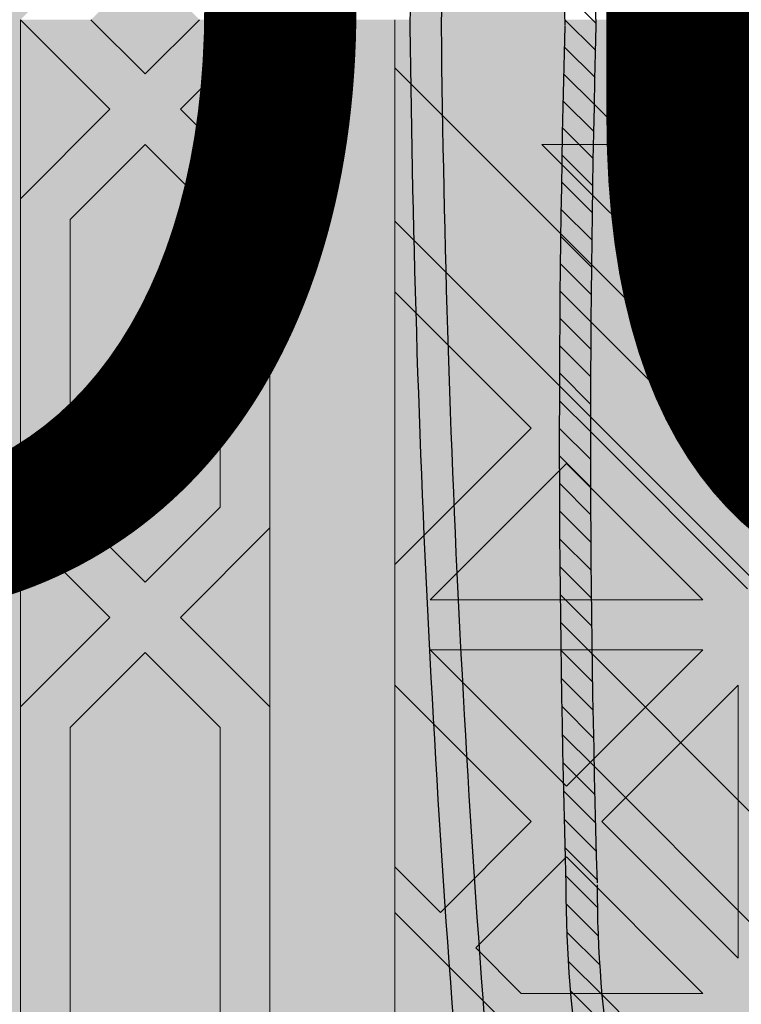
# Model space of a CAD drawing. Units: inches. Extents: x 844 to 2234, y 346 to 1084.
# Tile 71 of 93: x 1997.478 to 2001.166, y 696.335 to 701.365. Entities that reach past the tile are written whole.
import ezdxf

# ---------------------------------------------------------------- set-up
doc = ezdxf.new("R2010")
doc.units = ezdxf.units.IN
doc.header["$MEASUREMENT"] = 0
for name, color, linetype, lineweight in [('A-ANNO-DIMS', 2, 'Continuous', 18), ('furniture', 8, 'Continuous', 18), ('RA-AP-01$0$INT', 35, 'Continuous', 5)]:
    doc.layers.add(name, color=color, linetype=linetype, lineweight=lineweight)
doc.layers.add('RA-AP-01$0$FURN', color=3, linetype='Continuous')
doc.layers.add('RA-AP-01$0$WOOD', color=64, linetype='Continuous')
doc.styles.get("Standard").update_dxf_attribs({"font": 'arial.ttf'})
doc.dimstyles.get("Standard").update_dxf_attribs({"dimtxt": 6, "dimasz": 3, "dimexe": 0.18, "dimexo": 0.0625, "dimgap": 0.09, "dimtad": 0, "dimtih": 1, "dimtoh": 1, "dimdec": 1, "dimzin": 0, "dimdsep": 46, "dimlunit": 3, "dimtxsty": 'Standard', "dimblk": 'ARCHTICK', "dimcen": 0.09, "dimadec": 0, "dimazin": 0, "dimtfac": 1, "dimtdec": 1, "dimtofl": 0, "dimtmove": 0, "dimatfit": 3, "dimfxl": 1, "dimtolj": 1, "dimtzin": 0, "dimarcsym": 0})

# ---------------------------------------------------------------- blocks, each defined once
blk = doc.blocks.new('A$C18D01794')
at = {"layer": 'RA-AP-01$0$INT'}
h = blk.add_hatch(color=256, dxfattribs=at)
h.paths.add_polyline_path([(4.35521, -6.15671), (4.35521, -8.05671), (5.45521, -8.05671), (5.45521, -6.15671)])
h.paths.add_polyline_path([(4.40521, -8.00671), (4.40521, -6.20671), (5.40521, -6.20671), (5.40521, -8.00671)], flags=16)
h = blk.add_hatch(color=256, dxfattribs=at)
h.paths.add_polyline_path([(4.46935, -7.07085), (4.50521, -7.035), (4.50521, -7.10671)])
h.paths.add_polyline_path([(4.45521, -7.085), (4.47692, -7.10671), (4.43349, -7.10671)])
h.paths.add_polyline_path([(4.40521, -7.035), (4.44106, -7.07085), (4.40521, -7.10671)])
h.paths.add_polyline_path([(4.42521, -6.91146), (4.45521, -6.88146), (4.48521, -6.91146), (4.48521, -7.02671), (4.45521, -7.05671), (4.42521, -7.02671)])
h.paths.add_polyline_path([(4.50521, -6.83146), (4.50521, -6.90318), (4.46935, -6.86732)])
h.paths.add_polyline_path([(4.42521, -6.70793), (4.45521, -6.67793), (4.48521, -6.70793), (4.48521, -6.82318), (4.45521, -6.85318), (4.42521, -6.82318)])
h.paths.add_polyline_path([(4.42521, -6.50439), (4.45521, -6.47439), (4.48521, -6.50439), (4.48521, -6.61964), (4.45521, -6.64964), (4.42521, -6.61964)])
h.paths.add_polyline_path([(4.46935, -6.66378), (4.50521, -6.62793), (4.50521, -6.69964)])
h.paths.add_polyline_path([(4.40521, -6.62793), (4.44106, -6.66378), (4.40521, -6.69964)])
h.paths.add_polyline_path([(4.40521, -6.42439), (4.44106, -6.46025), (4.40521, -6.49611)])
h.paths.add_polyline_path([(4.46935, -6.46025), (4.50521, -6.42439), (4.50521, -6.49611)])
h.paths.add_polyline_path([(4.42521, -6.30085), (4.45521, -6.27085), (4.48521, -6.30085), (4.48521, -6.41611), (4.45521, -6.44611), (4.42521, -6.41611)])
h.paths.add_polyline_path([(4.42521, -6.22671), (4.47106, -6.22671), (4.42521, -6.27257)])
h.paths.add_polyline_path([(4.49935, -6.22671), (4.63606, -6.22671), (4.66606, -6.25671), (4.63606, -6.28671), (4.49935, -6.28671), (4.46935, -6.25671)])
h.paths.add_polyline_path([(4.68021, -6.27085), (4.71606, -6.30671), (4.64435, -6.30671)])
h.paths.add_polyline_path([(4.64435, -6.20671), (4.71606, -6.20671), (4.68021, -6.24257)])
h.paths.add_polyline_path([(4.72435, -6.22671), (4.86106, -6.22671), (4.89106, -6.25671), (4.86106, -6.28671), (4.72435, -6.28671), (4.69435, -6.25671)])
h.paths.add_polyline_path([(4.90521, -6.27085), (4.94106, -6.30671), (4.86935, -6.30671)])
h.paths.add_polyline_path([(4.86935, -6.20671), (4.94106, -6.20671), (4.90521, -6.24257)])
h.paths.add_polyline_path([(4.94935, -6.22671), (5.08606, -6.22671), (5.11606, -6.25671), (5.08606, -6.28671), (4.94935, -6.28671), (4.91935, -6.25671)])
h.paths.add_polyline_path([(5.13021, -6.27085), (5.16606, -6.30671), (5.09435, -6.30671)])
h.paths.add_polyline_path([(5.09435, -6.20671), (5.16606, -6.20671), (5.13021, -6.24257)])
h.paths.add_polyline_path([(5.17435, -6.22671), (5.31106, -6.22671), (5.34106, -6.25671), (5.31106, -6.28671), (5.17435, -6.28671), (5.14435, -6.25671)])
h.paths.add_polyline_path([(5.32521, -6.30085), (5.35521, -6.27085), (5.38521, -6.30085), (5.38521, -6.41611), (5.35521, -6.44611), (5.32521, -6.41611)])
h.paths.add_polyline_path([(5.33935, -6.22671), (5.38521, -6.22671), (5.38521, -6.27257)])
h.paths.add_polyline_path([(5.32521, -6.50439), (5.35521, -6.47439), (5.38521, -6.50439), (5.38521, -6.61964), (5.35521, -6.64964), (5.32521, -6.61964)])
h.paths.add_polyline_path([(5.30521, -6.42439), (5.34106, -6.46025), (5.30521, -6.49611)])
h.paths.add_polyline_path([(5.36935, -6.46025), (5.40521, -6.42439), (5.40521, -6.49611)])
h.paths.add_polyline_path([(5.40521, -6.62793), (5.40521, -6.69964), (5.36935, -6.66378)])
h.paths.add_polyline_path([(5.30521, -6.62793), (5.34106, -6.66378), (5.30521, -6.69964)])
h.paths.add_polyline_path([(5.32521, -6.70793), (5.35521, -6.67793), (5.38521, -6.70793), (5.38521, -6.82318), (5.35521, -6.85318), (5.32521, -6.82318)])
h.paths.add_polyline_path([(5.30521, -6.83146), (5.34106, -6.86732), (5.30521, -6.90318)])
h.paths.add_polyline_path([(5.32521, -6.91146), (5.35521, -6.88146), (5.38521, -6.91146), (5.38521, -7.02671), (5.35521, -7.05671), (5.32521, -7.02671)])
h.paths.add_polyline_path([(5.40458, -6.83209, 0.001218), (5.40521, -6.83231), (5.40521, -6.90318), (5.36935, -6.86732)])
h.paths.add_polyline_path([(5.36935, -7.07085), (5.40521, -7.035), (5.40521, -7.10671)])
h.paths.add_polyline_path([(5.35521, -7.085), (5.37692, -7.10671), (5.33349, -7.10671)])
h.paths.add_polyline_path([(5.30521, -7.035), (5.34106, -7.07085), (5.30521, -7.10671)])
h = blk.add_hatch(color=256, dxfattribs=at)
h.paths.add_polyline_path([(4.50521, -6.62793), (4.46935, -6.66378), (4.50521, -6.69964), (4.50521, -6.83146), (4.46935, -6.86732), (4.50521, -6.90318), (4.50521, -7.035), (4.46935, -7.07085), (4.50521, -7.10671), (4.47692, -7.10671), (4.45521, -7.085), (4.43349, -7.10671), (4.40521, -7.10671), (4.44106, -7.07085), (4.40521, -7.035), (4.40521, -6.90318), (4.44106, -6.86732), (4.40521, -6.83146), (4.40521, -6.69964), (4.44106, -6.66378), (4.40521, -6.62793), (4.40521, -6.49611), (4.44106, -6.46025), (4.40521, -6.42439), (4.40521, -6.20671), (4.64435, -6.20671), (4.68021, -6.24257), (4.71606, -6.20671), (4.86935, -6.20671), (4.90521, -6.24257), (4.94106, -6.20671), (5.09435, -6.20671), (5.13021, -6.24257), (5.16606, -6.20671), (5.40521, -6.20671), (5.40521, -6.42439), (5.36935, -6.46025), (5.40521, -6.49611), (5.40521, -6.62793), (5.36935, -6.66378), (5.40521, -6.69964), (5.40521, -6.83146), (5.36935, -6.86732), (5.40521, -6.90318), (5.40521, -7.035), (5.36935, -7.07085), (5.40521, -7.10671), (5.37692, -7.10671), (5.35521, -7.085), (5.33349, -7.10671), (5.30521, -7.10671), (5.34106, -7.07085), (5.30521, -7.035), (5.30521, -6.90318), (5.34106, -6.86732), (5.30521, -6.83146), (5.30521, -6.69964), (5.34106, -6.66378), (5.30521, -6.62793), (5.30521, -6.49611), (5.34106, -6.46025), (5.30521, -6.42439), (5.30521, -6.30671), (5.16606, -6.30671), (5.13021, -6.27085), (5.09435, -6.30671), (4.94106, -6.30671), (4.90521, -6.27085), (4.86935, -6.30671), (4.71606, -6.30671), (4.68021, -6.27085), (4.64435, -6.30671), (4.50521, -6.30671), (4.50521, -6.42439), (4.46935, -6.46025), (4.50521, -6.49611)])
h.paths.add_polyline_path([(4.48521, -6.50439), (4.45521, -6.47439), (4.42521, -6.50439), (4.42521, -6.61964), (4.45521, -6.64964), (4.48521, -6.61964)], flags=16)
h.paths.add_polyline_path([(4.45521, -6.44611), (4.48521, -6.41611), (4.48521, -6.30085), (4.45521, -6.27085), (4.42521, -6.30085), (4.42521, -6.41611)], flags=16)
h.paths.add_polyline_path([(4.45521, -6.67793), (4.42521, -6.70793), (4.42521, -6.82318), (4.45521, -6.85318), (4.48521, -6.82318), (4.48521, -6.70793)], flags=16)
h.paths.add_polyline_path([(4.49935, -6.28671), (4.63606, -6.28671), (4.66606, -6.25671), (4.63606, -6.22671), (4.49935, -6.22671), (4.46935, -6.25671)], flags=16)
h.paths.add_polyline_path([(4.42521, -6.27257), (4.47106, -6.22671), (4.42521, -6.22671)], flags=16)
h.paths.add_polyline_path([(4.45521, -6.88146), (4.42521, -6.91146), (4.42521, -7.02671), (4.45521, -7.05671), (4.48521, -7.02671), (4.48521, -6.91146)], flags=16)
h.paths.add_polyline_path([(4.72435, -6.28671), (4.86106, -6.28671), (4.89106, -6.25671), (4.86106, -6.22671), (4.72435, -6.22671), (4.69435, -6.25671)], flags=16)
h.paths.add_polyline_path([(4.91935, -6.25671), (4.94935, -6.28671), (5.08606, -6.28671), (5.11606, -6.25671), (5.08606, -6.22671), (4.94935, -6.22671)], flags=16)
h.paths.add_polyline_path([(5.14435, -6.25671), (5.17435, -6.28671), (5.31106, -6.28671), (5.34106, -6.25671), (5.31106, -6.22671), (5.17435, -6.22671)], flags=16)
h.paths.add_polyline_path([(5.32521, -6.61964), (5.35521, -6.64964), (5.38521, -6.61964), (5.38521, -6.50439), (5.35521, -6.47439), (5.32521, -6.50439)], flags=16)
h.paths.add_polyline_path([(5.32521, -6.41611), (5.35521, -6.44611), (5.38521, -6.41611), (5.38521, -6.30085), (5.35521, -6.27085), (5.32521, -6.30085)], flags=16)
h.paths.add_polyline_path([(5.32521, -6.70793), (5.32521, -6.82318), (5.35521, -6.85318), (5.38521, -6.82318), (5.38521, -6.70793), (5.35521, -6.67793)], flags=16)
h.paths.add_polyline_path([(5.32521, -6.91146), (5.32521, -7.02671), (5.35521, -7.05671), (5.38521, -7.02671), (5.38521, -6.91146), (5.35521, -6.88146)], flags=16)
h.paths.add_polyline_path([(5.33935, -6.22671), (5.38521, -6.27257), (5.38521, -6.22671)], flags=16)
blk.add_hatch(color=256, dxfattribs=at).paths.add_polyline_path([(4.50521, -6.30671), (5.30521, -6.30671), (5.30521, -7.10671), (5.25521, -7.10671), (5.25521, -6.35671), (4.55521, -6.35671), (4.55521, -7.10671), (4.50521, -7.10671)])
h = blk.add_hatch(color=256, dxfattribs=at)
h.paths.add_polyline_path([(4.58592, -6.35671), (4.55521, -6.35671), (4.55521, -6.38742), (4.8745, -6.70671), (4.90521, -6.676)])
h.paths.add_polyline_path([(5.25521, -6.38742), (5.25521, -6.35671), (5.2245, -6.35671), (4.90521, -6.676), (4.93592, -6.70671)])
h.paths.add_polyline_path([(4.93592, -6.70671), (4.90521, -6.73742), (5.25521, -7.08742), (5.25521, -7.026)])
h.paths.add_polyline_path([(4.55521, -7.026), (4.55521, -7.08742), (4.90521, -6.73742), (4.8745, -6.70671)])
h = blk.add_hatch(color=256, dxfattribs=at)
h.paths.add_polyline_path([(4.58592, -6.35671), (4.6142, -6.35671), (4.66885, -6.41136), (4.72349, -6.35671), (4.77177, -6.35671), (4.82642, -6.41136), (4.86278, -6.375), (4.8445, -6.35671), (4.86278, -6.35671), (4.90521, -6.39914), (4.94763, -6.35671), (4.96592, -6.35671), (4.94763, -6.375), (4.98399, -6.41136), (5.03864, -6.35671), (5.08692, -6.35671), (5.14157, -6.41136), (5.19621, -6.35671), (5.2245, -6.35671), (4.90521, -6.676)])
h.paths.add_polyline_path([(4.89521, -6.63772), (4.89521, -6.52843), (4.84056, -6.58307)], flags=16)
h.paths.add_polyline_path([(4.91521, -6.63772), (4.96985, -6.58307), (4.91521, -6.52843)], flags=16)
h.paths.add_polyline_path([(4.82642, -6.56893), (4.88106, -6.51429), (4.77177, -6.51429)], flags=16)
h.paths.add_polyline_path([(4.98399, -6.56893), (5.03864, -6.51429), (4.92935, -6.51429)], flags=16)
h.paths.add_polyline_path([(4.88106, -6.49429), (4.82642, -6.43964), (4.77177, -6.49429)], flags=16)
h.paths.add_polyline_path([(4.92935, -6.49429), (5.03864, -6.49429), (4.98399, -6.43964)], flags=16)
h.paths.add_polyline_path([(4.89521, -6.48014), (4.89521, -6.40742), (4.87692, -6.38914), (4.84056, -6.4255)], flags=16)
h.paths.add_polyline_path([(4.91521, -6.48014), (4.96985, -6.4255), (4.93349, -6.38914), (4.91521, -6.40742)], flags=16)
h.paths.add_polyline_path([(4.75763, -6.48014), (4.81228, -6.4255), (4.75763, -6.37085)], flags=16)
h.paths.add_polyline_path([(4.73763, -6.48014), (4.73763, -6.37085), (4.68299, -6.4255)], flags=16)
h.paths.add_polyline_path([(5.05278, -6.48014), (5.05278, -6.37085), (4.99814, -6.4255)], flags=16)
h.paths.add_polyline_path([(5.07278, -6.48014), (5.12742, -6.4255), (5.07278, -6.37085)], flags=16)
h.paths.add_polyline_path([(4.93592, -6.70671), (5.25521, -6.38742), (5.25521, -6.41571), (5.20056, -6.47035), (5.25521, -6.525), (5.25521, -6.57328), (5.20056, -6.62793), (5.23692, -6.66429), (5.25521, -6.646), (5.25521, -6.66429), (5.21278, -6.70671), (5.25521, -6.74914), (5.25521, -6.76742), (5.23692, -6.74914), (5.20056, -6.7855), (5.25521, -6.84014), (5.25521, -6.88843), (5.20056, -6.94307), (5.25521, -6.99772), (5.25521, -7.026)])
h.paths.add_polyline_path([(5.04299, -6.7855), (5.09763, -6.84014), (5.09763, -6.73085)], flags=16)
h.paths.add_polyline_path([(5.02885, -6.77136), (5.08349, -6.71671), (4.9742, -6.71671)], flags=16)
h.paths.add_polyline_path([(5.11763, -6.84014), (5.17228, -6.7855), (5.11763, -6.73085)], flags=16)
h.paths.add_polyline_path([(5.08349, -6.69671), (5.02885, -6.64207), (4.9742, -6.69671)], flags=16)
h.paths.add_polyline_path([(5.13177, -6.85429), (5.18642, -6.79964), (5.24106, -6.85429)], flags=17)
h.paths.add_polyline_path([(5.13177, -6.71671), (5.18642, -6.77136), (5.22278, -6.735), (5.2045, -6.71671)], flags=16)
h.paths.add_polyline_path([(5.09763, -6.68257), (5.09763, -6.57328), (5.04299, -6.62793)], flags=16)
h.paths.add_polyline_path([(5.13177, -6.87429), (5.24106, -6.87429), (5.18642, -6.92893)], flags=17)
h.paths.add_polyline_path([(5.13177, -6.69671), (5.2045, -6.69671), (5.22278, -6.67843), (5.18642, -6.64207)], flags=16)
h.paths.add_polyline_path([(5.11763, -6.68257), (5.17228, -6.62793), (5.11763, -6.57328)], flags=16)
h.paths.add_polyline_path([(5.18642, -6.61378), (5.24106, -6.55914), (5.13177, -6.55914)], flags=16)
h.paths.add_polyline_path([(5.13177, -6.53914), (5.24106, -6.53914), (5.18642, -6.48449)], flags=16)
h.paths.add_polyline_path([(5.25521, -7.08742), (5.25521, -7.10671), (4.55521, -7.10671), (4.55521, -7.08742), (4.90521, -6.73742)])
h.paths.add_polyline_path([(4.98399, -6.84449), (4.92935, -6.89914), (5.03864, -6.89914)], flags=16)
h.paths.add_polyline_path([(4.96985, -6.83035), (4.91521, -6.77571), (4.91521, -6.885)], flags=16)
h.paths.add_polyline_path([(4.92935, -6.91914), (4.98399, -6.97378), (5.03864, -6.91914)], flags=16)
h.paths.add_polyline_path([(5.05278, -6.93328), (4.99814, -6.98793), (5.05278, -7.04257)], flags=16)
h.paths.add_polyline_path([(5.07278, -6.93328), (5.07278, -7.04257), (5.12742, -6.98793)], flags=16)
h.paths.add_polyline_path([(4.89521, -6.77571), (4.84056, -6.83035), (4.89521, -6.885)], flags=16)
h.paths.add_polyline_path([(4.91521, -6.93328), (4.91521, -7.006), (4.93349, -7.02429), (4.96985, -6.98793)], flags=16)
h.paths.add_polyline_path([(4.88106, -6.89914), (4.82642, -6.84449), (4.77177, -6.89914)], flags=16)
h.paths.add_polyline_path([(4.89521, -6.93328), (4.84056, -6.98793), (4.87692, -7.02429), (4.89521, -7.006)], flags=16)
h.paths.add_polyline_path([(4.98399, -7.00207), (4.94763, -7.03843), (4.96592, -7.05671), (5.03864, -7.05671)], flags=16)
h.paths.add_polyline_path([(4.88106, -6.91914), (4.77177, -6.91914), (4.82642, -6.97378)], flags=16)
h.paths.add_polyline_path([(4.90521, -7.01429), (4.86278, -7.05671), (4.94763, -7.05671)], flags=16)
h.paths.add_polyline_path([(5.14157, -7.00207), (5.08692, -7.05671), (5.19621, -7.05671)], flags=16)
h.paths.add_polyline_path([(4.82642, -7.00207), (4.77177, -7.05671), (4.8445, -7.05671), (4.86278, -7.03843)], flags=16)
h.paths.add_polyline_path([(4.81228, -6.98793), (4.75763, -6.93328), (4.75763, -7.04257)], flags=16)
h.paths.add_polyline_path([(4.73763, -6.93328), (4.68299, -6.98793), (4.73763, -7.04257)], flags=16)
h.paths.add_polyline_path([(4.72349, -7.05671), (4.66885, -7.00207), (4.6142, -7.05671)], flags=16)
h.paths.add_polyline_path([(4.59763, -6.70671), (4.55521, -6.66429), (4.55521, -6.646), (4.57349, -6.66429), (4.60985, -6.62793), (4.55521, -6.57328), (4.55521, -6.525), (4.60985, -6.47035), (4.55521, -6.41571), (4.55521, -6.38742), (4.8745, -6.70671), (4.55521, -7.026), (4.55521, -6.99772), (4.60985, -6.94307), (4.55521, -6.88843), (4.55521, -6.84014), (4.60985, -6.7855), (4.57349, -6.74914), (4.55521, -6.76742), (4.55521, -6.74914)])
h.paths.add_polyline_path([(4.71278, -6.73085), (4.71278, -6.84014), (4.76742, -6.7855)], flags=16)
h.paths.add_polyline_path([(4.72692, -6.71671), (4.78157, -6.77136), (4.83621, -6.71671)], flags=16)
h.paths.add_polyline_path([(4.69278, -6.73085), (4.63814, -6.7855), (4.69278, -6.84014)], flags=16)
h.paths.add_polyline_path([(4.72692, -6.69671), (4.83621, -6.69671), (4.78157, -6.64207)], flags=16)
h.paths.add_polyline_path([(4.67864, -6.71671), (4.60592, -6.71671), (4.58763, -6.735), (4.62399, -6.77136)], flags=16)
h.paths.add_polyline_path([(4.71278, -6.68257), (4.76742, -6.62793), (4.71278, -6.57328)], flags=16)
h.paths.add_polyline_path([(4.67864, -6.69671), (4.62399, -6.64207), (4.58763, -6.67843), (4.60592, -6.69671)], flags=16)
h.paths.add_polyline_path([(4.69278, -6.68257), (4.69278, -6.57328), (4.63814, -6.62793)], flags=16)
h.paths.add_polyline_path([(4.62399, -6.79964), (4.67864, -6.85429), (4.56935, -6.85429)], flags=17)
h.paths.add_polyline_path([(4.62399, -6.61378), (4.67864, -6.55914), (4.56935, -6.55914)], flags=16)
h.paths.add_polyline_path([(4.67864, -6.87429), (4.62399, -6.92893), (4.56935, -6.87429)], flags=17)
h.paths.add_polyline_path([(4.67864, -6.53914), (4.62399, -6.48449), (4.56935, -6.53914)], flags=16)
h = blk.add_hatch(color=256, dxfattribs=at)
h.paths.add_polyline_path([(5.02885, -6.64207), (4.9742, -6.69671), (5.08349, -6.69671)])
h.paths.add_polyline_path([(4.9742, -6.71671), (5.02885, -6.77136), (5.08349, -6.71671)])
h.paths.add_polyline_path([(5.04299, -6.7855), (5.09763, -6.84014), (5.09763, -6.73085)])
h.paths.add_polyline_path([(5.11763, -6.73085), (5.11763, -6.84014), (5.17228, -6.7855)])
h.paths.add_polyline_path([(5.13177, -6.71671), (5.18642, -6.77136), (5.22278, -6.735), (5.2045, -6.71671)])
h.paths.add_polyline_path([(5.23692, -6.74914), (5.20056, -6.7855), (5.25521, -6.84014), (5.25521, -6.76742)])
h.paths.add_polyline_path([(5.18642, -6.79964), (5.13177, -6.85429), (5.24106, -6.85429)])
h.paths.add_polyline_path([(5.13177, -6.87429), (5.18642, -6.92893), (5.24106, -6.87429)])
h.paths.add_polyline_path([(5.20056, -6.94307), (5.25521, -6.99772), (5.25521, -6.88843)])
h.paths.add_polyline_path([(5.21278, -6.70671), (5.25521, -6.74914), (5.25521, -6.66429)])
h.paths.add_polyline_path([(5.13177, -6.69671), (5.2045, -6.69671), (5.22278, -6.67843), (5.18642, -6.64207)])
h.paths.add_polyline_path([(5.11763, -6.57328), (5.11763, -6.68257), (5.17228, -6.62793)])
h.paths.add_polyline_path([(5.04299, -6.62793), (5.09763, -6.68257), (5.09763, -6.57328)])
h.paths.add_polyline_path([(5.13177, -6.55914), (5.18642, -6.61378), (5.24106, -6.55914)])
h.paths.add_polyline_path([(5.20056, -6.62793), (5.23692, -6.66429), (5.25521, -6.646), (5.25521, -6.57328)])
h.paths.add_polyline_path([(5.18642, -6.48449), (5.13177, -6.53914), (5.24106, -6.53914)])
h.paths.add_polyline_path([(5.20056, -6.47035), (5.25521, -6.525), (5.25521, -6.41571)])
h = blk.add_hatch(color=256, dxfattribs=at)
h.paths.add_polyline_path([(4.89521, -6.77571), (4.84056, -6.83035), (4.89521, -6.885)])
h.paths.add_polyline_path([(4.91521, -6.885), (4.96985, -6.83035), (4.91521, -6.77571)])
h.paths.add_polyline_path([(5.03864, -6.89914), (4.98399, -6.84449), (4.92935, -6.89914)])
h.paths.add_polyline_path([(4.92935, -6.91914), (4.98399, -6.97378), (5.03864, -6.91914)])
h.paths.add_polyline_path([(4.91521, -6.93328), (4.91521, -7.006), (4.93349, -7.02429), (4.96985, -6.98793)])
h.paths.add_polyline_path([(5.03864, -7.05671), (4.98399, -7.00207), (4.94763, -7.03843), (4.96592, -7.05671)])
h.paths.add_polyline_path([(5.05278, -7.04257), (5.05278, -6.93328), (4.99814, -6.98793)])
h.paths.add_polyline_path([(5.07278, -7.04257), (5.12742, -6.98793), (5.07278, -6.93328)])
h.paths.add_polyline_path([(5.14157, -7.00207), (5.08692, -7.05671), (5.19621, -7.05671)])
h.paths.add_polyline_path([(4.94763, -7.05671), (4.90521, -7.01429), (4.86278, -7.05671)])
h.paths.add_polyline_path([(4.84056, -6.98793), (4.87692, -7.02429), (4.89521, -7.006), (4.89521, -6.93328)])
h.paths.add_polyline_path([(4.88106, -6.91914), (4.77177, -6.91914), (4.82642, -6.97378)])
h.paths.add_polyline_path([(4.88106, -6.89914), (4.82642, -6.84449), (4.77177, -6.89914)])
h.paths.add_polyline_path([(4.75763, -7.04257), (4.81228, -6.98793), (4.75763, -6.93328)])
h.paths.add_polyline_path([(4.82642, -7.00207), (4.77177, -7.05671), (4.8445, -7.05671), (4.86278, -7.03843)])
h.paths.add_polyline_path([(4.73763, -7.04257), (4.73763, -6.93328), (4.68299, -6.98793)])
h.paths.add_polyline_path([(4.66885, -7.00207), (4.6142, -7.05671), (4.72349, -7.05671)])
h = blk.add_hatch(color=256, dxfattribs=at)
h.paths.add_polyline_path([(4.46935, -7.14257), (4.50521, -7.17843), (4.50521, -7.10671)])
h.paths.add_polyline_path([(4.45521, -7.12843), (4.47692, -7.10671), (4.43349, -7.10671)])
h.paths.add_polyline_path([(4.40521, -7.17843), (4.44106, -7.14257), (4.40521, -7.10671)])
h.paths.add_polyline_path([(4.42521, -7.30196), (4.45521, -7.33196), (4.48521, -7.30196), (4.48521, -7.18671), (4.45521, -7.15671), (4.42521, -7.18671)])
h.paths.add_polyline_path([(4.50521, -7.38196), (4.50521, -7.31025), (4.46935, -7.34611)])
h.paths.add_polyline_path([(4.42521, -7.5055), (4.45521, -7.5355), (4.48521, -7.5055), (4.48521, -7.39025), (4.45521, -7.36025), (4.42521, -7.39025)])
h.paths.add_polyline_path([(4.42521, -7.70903), (4.45521, -7.73903), (4.48521, -7.70903), (4.48521, -7.59378), (4.45521, -7.56378), (4.42521, -7.59378)])
h.paths.add_polyline_path([(4.46935, -7.54964), (4.50521, -7.5855), (4.50521, -7.51378)])
h.paths.add_polyline_path([(4.40521, -7.5855), (4.44106, -7.54964), (4.40521, -7.51378)])
h.paths.add_polyline_path([(4.40521, -7.78903), (4.44106, -7.75318), (4.40521, -7.71732)])
h.paths.add_polyline_path([(4.46935, -7.75318), (4.50521, -7.78903), (4.50521, -7.71732)])
h.paths.add_polyline_path([(4.42521, -7.91257), (4.45521, -7.94257), (4.48521, -7.91257), (4.48521, -7.79732), (4.45521, -7.76732), (4.42521, -7.79732)])
h.paths.add_polyline_path([(4.42521, -7.98671), (4.47106, -7.98671), (4.42521, -7.94085)])
h.paths.add_polyline_path([(4.49935, -7.98671), (4.63606, -7.98671), (4.66606, -7.95671), (4.63606, -7.92671), (4.49935, -7.92671), (4.46935, -7.95671)])
h.paths.add_polyline_path([(4.68021, -7.94257), (4.71606, -7.90671), (4.64435, -7.90671)])
h.paths.add_polyline_path([(4.64435, -8.00671), (4.71606, -8.00671), (4.68021, -7.97085)])
h.paths.add_polyline_path([(4.72435, -7.98671), (4.86106, -7.98671), (4.89106, -7.95671), (4.86106, -7.92671), (4.72435, -7.92671), (4.69435, -7.95671)])
h.paths.add_polyline_path([(4.90521, -7.94257), (4.94106, -7.90671), (4.86935, -7.90671)])
h.paths.add_polyline_path([(4.86935, -8.00671), (4.94106, -8.00671), (4.90521, -7.97085)])
h.paths.add_polyline_path([(4.94935, -7.98671), (5.08606, -7.98671), (5.11606, -7.95671), (5.08606, -7.92671), (4.94935, -7.92671), (4.91935, -7.95671)])
h.paths.add_polyline_path([(5.13021, -7.94257), (5.16606, -7.90671), (5.09435, -7.90671)])
h.paths.add_polyline_path([(5.09435, -8.00671), (5.16606, -8.00671), (5.13021, -7.97085)])
h.paths.add_polyline_path([(5.17435, -7.98671), (5.31106, -7.98671), (5.34106, -7.95671), (5.31106, -7.92671), (5.17435, -7.92671), (5.14435, -7.95671)])
h.paths.add_polyline_path([(5.32521, -7.91257), (5.35521, -7.94257), (5.38521, -7.91257), (5.38521, -7.79732), (5.35521, -7.76732), (5.32521, -7.79732)])
h.paths.add_polyline_path([(5.33935, -7.98671), (5.38521, -7.98671), (5.38521, -7.94085)])
h.paths.add_polyline_path([(5.32521, -7.70903), (5.35521, -7.73903), (5.38521, -7.70903), (5.38521, -7.59378), (5.35521, -7.56378), (5.32521, -7.59378)])
h.paths.add_polyline_path([(5.30521, -7.78903), (5.34106, -7.75318), (5.30521, -7.71732)])
h.paths.add_polyline_path([(5.36935, -7.75318), (5.40521, -7.78903), (5.40521, -7.71732)])
h.paths.add_polyline_path([(5.40521, -7.5855), (5.40521, -7.51378), (5.36935, -7.54964)])
h.paths.add_polyline_path([(5.30521, -7.5855), (5.34106, -7.54964), (5.30521, -7.51378)])
h.paths.add_polyline_path([(5.32521, -7.5055), (5.35521, -7.5355), (5.38521, -7.5055), (5.38521, -7.39025), (5.35521, -7.36025), (5.32521, -7.39025)])
h.paths.add_polyline_path([(5.30521, -7.38196), (5.34106, -7.34611), (5.30521, -7.31025)])
h.paths.add_polyline_path([(5.32521, -7.30196), (5.35521, -7.33196), (5.38521, -7.30196), (5.38521, -7.18671), (5.35521, -7.15671), (5.32521, -7.18671)])
h.paths.add_polyline_path([(5.40458, -7.38134, -0.001218), (5.40521, -7.38111), (5.40521, -7.31025), (5.36935, -7.34611)])
h.paths.add_polyline_path([(5.36935, -7.14257), (5.40521, -7.17843), (5.40521, -7.10671)])
h.paths.add_polyline_path([(5.35521, -7.12843), (5.37692, -7.10671), (5.33349, -7.10671)])
h.paths.add_polyline_path([(5.30521, -7.17843), (5.34106, -7.14257), (5.30521, -7.10671)])
for p, q in [((5.25521, -7.10671), (5.25521, -6.35671)), ((5.25521, -6.74914), (5.25521, -6.66429)), ((4.93592, -6.70671), (5.25521, -7.026)), ((5.21278, -6.70671), (5.25521, -6.74914)), ((5.32521, -6.82318), (5.32521, -6.70793)), ((5.38521, -6.82318), (5.38521, -6.70793)), ((5.13177, -6.71671), (5.18642, -6.77136)), ((5.2045, -6.71671), (5.13177, -6.71671)), ((5.2045, -6.71671), (5.22278, -6.735)), ((5.11763, -6.73085), (5.17228, -6.7855)), ((5.11763, -6.84014), (5.11763, -6.73085)), ((5.18642, -6.77136), (5.22278, -6.735)), ((4.90521, -6.73742), (5.25521, -7.08742)), ((5.20056, -6.7855), (5.23692, -6.74914)), ((5.25521, -6.76742), (5.23692, -6.74914)), ((5.23692, -6.74914), (5.25521, -6.76742)), ((5.25521, -6.76742), (5.25521, -6.84014)), ((5.11763, -6.84014), (5.17228, -6.7855)), ((5.25521, -6.84014), (5.20056, -6.7855)), ((5.13177, -6.85429), (5.18642, -6.79964)), ((5.24106, -6.85429), (5.18642, -6.79964)), ((5.32521, -6.82318), (5.35521, -6.85318)), ((5.38521, -6.82318), (5.35521, -6.85318)), ((5.30521, -6.83146), (5.34106, -6.86732)), ((5.40521, -6.83146), (5.36935, -6.86732)), ((5.13177, -6.85429), (5.24106, -6.85429)), ((5.30521, -6.90318), (5.34106, -6.86732)), ((5.40521, -6.90318), (5.36935, -6.86732)), ((5.13177, -6.87429), (5.24106, -6.87429)), ((5.18642, -6.92893), (5.13177, -6.87429)), ((5.24106, -6.87429), (5.18642, -6.92893)), ((5.32521, -6.91146), (5.35521, -6.88146)), ((5.38521, -6.91146), (5.35521, -6.88146)), ((5.25521, -6.88843), (5.20056, -6.94307)), ((5.25521, -6.88843), (5.25521, -6.99772)), ((5.32521, -6.91146), (5.32521, -7.02671)), ((5.38521, -6.91146), (5.38521, -7.02671)), ((5.12742, -6.98793), (5.07278, -6.93328)), ((5.25521, -6.99772), (5.20056, -6.94307)), ((5.07278, -7.04257), (5.12742, -6.98793)), ((5.08692, -7.05671), (5.14157, -7.00207)), ((5.19621, -7.05671), (5.14157, -7.00207)), ((5.32521, -7.02671), (5.35521, -7.05671)), ((5.38521, -7.02671), (5.35521, -7.05671)), ((5.30521, -7.035), (5.34106, -7.07085)), ((5.40521, -7.035), (5.36935, -7.07085)), ((5.08692, -7.05671), (5.19621, -7.05671)), ((5.34106, -7.07085), (5.30521, -7.10671)), ((5.36935, -7.07085), (5.40521, -7.10671)), ((5.35521, -7.085), (5.33349, -7.10671)), ((5.35521, -7.085), (5.37692, -7.10671))]:
    blk.add_line(p, q, dxfattribs=at)
for points in [[(5.40521, -7.10671), (5.40521, -6.20671)], [(5.30521, -7.10671), (5.30521, -6.30671), (4.50521, -6.30671), (4.50521, -7.10671)]]:
    blk.add_lwpolyline(points, dxfattribs=at)
blk = doc.blocks.new('A$C32926AE1')
at = {"layer": 'RA-AP-01$0$WOOD'}
h = blk.add_hatch(color=256, dxfattribs=at)
h.dxf.hatch_style = 1
h.paths.add_polyline_path([(5.15743, 4.57348, -0.100949), (5.1554, 4.59337, -0.184266), (5.17225, 4.6388, 0.205661), (5.17956, 4.66132, 0.361434), (5.13435, 4.70652, 0.205661), (5.11183, 4.69921, -0.184266), (5.0664, 4.68237, -0.105531), (5.04566, 4.68467, 0.156764), (4.76389, 4.68467, -0.105531), (4.74314, 4.68237, -0.184266), (4.69771, 4.69921, 0.205661), (4.67519, 4.70652, 0.361434), (4.62998, 4.66132, 0.205661), (4.63729, 4.6388, -0.184266), (4.65414, 4.59337, -0.100949), (4.65211, 4.57348, 0.02141), (4.62975, 4.15671, 0.02141), (4.65211, 3.73994, -0.100949), (4.65414, 3.72006, -0.184266), (4.63729, 3.67463, 0.205661), (4.62998, 3.65211, 0.361434), (4.67519, 3.6069, 0.205661), (4.69771, 3.61421, -0.184266), (4.74314, 3.63106, -0.105531), (4.76389, 3.62875, 0.156764), (5.04566, 3.62875, -0.105531), (5.0664, 3.63106, -0.184266), (5.11183, 3.61421, 0.205661), (5.13435, 3.6069, 0.361434), (5.17956, 3.65211, 0.205661), (5.17225, 3.67463, -0.184266), (5.1554, 3.72006, -0.100949), (5.15743, 3.73994, 0.02141), (5.17979, 4.15671, 0.02141)])
h.paths.add_polyline_path([(4.63975, 4.15671, 0.021354), (4.66197, 3.74189, -0.094076), (4.66414, 3.71961, -0.182482), (4.64481, 3.66804, 0.205661), (4.63994, 3.65302, 0.361434), (4.67611, 3.61686, 0.205661), (4.69112, 3.62173, -0.182482), (4.7427, 3.64106, -0.102989), (4.76699, 3.63826, 0.156709), (5.04255, 3.63826, -0.102989), (5.06685, 3.64106, -0.182482), (5.11842, 3.62173, 0.205661), (5.13344, 3.61686, 0.361434), (5.1696, 3.65302, 0.205661), (5.16473, 3.66804, -0.182482), (5.1454, 3.71961, -0.094076), (5.14757, 3.74189, 0.021354), (5.16979, 4.15671, 0.021354), (5.14757, 4.57154, -0.094076), (5.1454, 4.59381, -0.182482), (5.16473, 4.64539, 0.205661), (5.1696, 4.6604, 0.361434), (5.13344, 4.69657, 0.205661), (5.11842, 4.69169, -0.182482), (5.06685, 4.67236, -0.102989), (5.04255, 4.67517, 0.156709), (4.76699, 4.67517, -0.102989), (4.7427, 4.67236, -0.182482), (4.69112, 4.69169, 0.205661), (4.67611, 4.69657, 0.361434), (4.63994, 4.6604, 0.205661), (4.64481, 4.64539, -0.182482), (4.66414, 4.59381, -0.094076), (4.66197, 4.57154, 0.021354)], flags=16)
h.paths.add_polyline_path([(5.12979, 4.43217, -0.014166), (5.13015, 4.15693, -0.014166), (5.12979, 3.88169, -0.078525), (5.1098, 3.75514, 0.094597), (5.10541, 3.7179, 0.104317), (5.11607, 3.67039, 0.104317), (5.06856, 3.68105, 0.094597), (5.03132, 3.67666, -0.158024), (4.77823, 3.67666, 0.094597), (4.74098, 3.68105, 0.104317), (4.69347, 3.67039, 0.104317), (4.70413, 3.7179, 0.094597), (4.69975, 3.75514, -0.078525), (4.67975, 3.88169, -0.014166), (4.67939, 4.15693, -0.014166), (4.67975, 4.43217, -0.078525), (4.69975, 4.55871, 0.094597), (4.70413, 4.59596, 0.104317), (4.69347, 4.64347, 0.104317), (4.74098, 4.6328, 0.094597), (4.77823, 4.63719, -0.158024), (5.03132, 4.63719, 0.094597), (5.06856, 4.6328, 0.104317), (5.11607, 4.64347, 0.104317), (5.10541, 4.59596, 0.094597), (5.1098, 4.55871, -0.078525)], flags=0)
h.paths.add_polyline_path([(5.11979, 4.43226, -0.0142), (5.12016, 4.15693, -0.0142), (5.11979, 3.8816, -0.078489), (5.10027, 3.75819, 0.094014), (5.09541, 3.71748, 0.060627), (5.09962, 3.68684, 0.060627), (5.06898, 3.69105, 0.094014), (5.02827, 3.68619, -0.158071), (4.78127, 3.68619, 0.094014), (4.74056, 3.69105, 0.060627), (4.70993, 3.68684, 0.060627), (4.71413, 3.71748, 0.094014), (4.70927, 3.75819, -0.078489), (4.68975, 3.8816, -0.0142), (4.68939, 4.15693, -0.0142), (4.68975, 4.43226, -0.078489), (4.70927, 4.55566, 0.094014), (4.71413, 4.59638, 0.060627), (4.70993, 4.62701, 0.060627), (4.74056, 4.62281, 0.094014), (4.78127, 4.62767, -0.158071), (5.02827, 4.62767, 0.094014), (5.06898, 4.62281, 0.060627), (5.09962, 4.62701, 0.060627), (5.09541, 4.59638, 0.094014), (5.10027, 4.55566, -0.078489)], flags=0)
h.paths.add_polyline_path([(5.06979, 4.43022, -0.014242), (5.07017, 4.15693, -0.014242), (5.06979, 3.88364, -0.080061), (5.05266, 3.77346, 0.052642), (5.04591, 3.74055, 0.052642), (5.013, 3.7338, -0.158303), (4.79655, 3.7338, 0.052642), (4.76363, 3.74055, 0.052642), (4.75688, 3.77346, -0.080061), (4.73975, 3.88364, -0.014242), (4.73937, 4.15693, -0.014242), (4.73975, 4.43022, -0.080061), (4.75688, 4.54039, 0.052642), (4.76363, 4.5733, 0.052642), (4.79655, 4.58006, -0.158303), (5.013, 4.58006, 0.052642), (5.04591, 4.5733, 0.052642), (5.05266, 4.54039, -0.080061)], flags=0)
h.paths.add_polyline_path([(5.04979, 4.43038, -0.01431), (5.05018, 4.15693, -0.01431), (5.04979, 3.88347, -0.080069), (5.03362, 3.77958, 0.030626), (5.02824, 3.75822, 0.030626), (5.00688, 3.75284, -0.158398), (4.80266, 3.75284, 0.030626), (4.7813, 3.75822, 0.030626), (4.77592, 3.77958, -0.080069), (4.75975, 3.88347, -0.01431), (4.75936, 4.15693, -0.01431), (4.75975, 4.43038, -0.080069), (4.77592, 4.53427, 0.030626), (4.7813, 4.55564, 0.030626), (4.80266, 4.56102, -0.158398), (5.00688, 4.56102, 0.030626), (5.02824, 4.55564, 0.030626), (5.03362, 4.53427, -0.080069)], flags=0)
h.paths.add_polyline_path([(4.99977, 4.42817, -0.014344), (5.0002, 4.15693, -0.014344), (4.99977, 3.88568, -0.078464), (4.98736, 3.7991, -0.150605), (4.82219, 3.7991, -0.078464), (4.80978, 3.88568, -0.014344), (4.80934, 4.15693, -0.014344), (4.80978, 4.42817, -0.078464), (4.82219, 4.51475, -0.150605), (4.98736, 4.51475, -0.078464)], flags=0)
h.paths.add_polyline_path([(4.97976, 4.42764, -0.014377), (4.98021, 4.15693, -0.014377), (4.97976, 3.88621, -0.068924), (4.97118, 3.81528, -0.129665), (4.83836, 3.81528, -0.068924), (4.82979, 3.88621, -0.014377), (4.82934, 4.15693, -0.014377), (4.82979, 4.42764, -0.068924), (4.83836, 4.49858, -0.129665), (4.97118, 4.49858, -0.068924)], flags=0)
h = blk.add_hatch(color=256, dxfattribs=at)
h.dxf.hatch_style = 1
h.paths.add_polyline_path([(5.1454, 4.59381, -0.182482), (5.16473, 4.64539, 0.205661), (5.1696, 4.6604, 0.361434), (5.13344, 4.69657, 0.205661), (5.11842, 4.69169, -0.182482), (5.06685, 4.67236, -0.102989), (5.04255, 4.67517, 0.156709), (4.76699, 4.67517, -0.102989), (4.7427, 4.67236, -0.182482), (4.69112, 4.69169, 0.205661), (4.67611, 4.69657, 0.361434), (4.63994, 4.6604, 0.205661), (4.64481, 4.64539, -0.182482), (4.66414, 4.59381, -0.094076), (4.66197, 4.57154, 0.021354), (4.63975, 4.15671, 0.021354), (4.66197, 3.74189, -0.094076), (4.66414, 3.71961, -0.182482), (4.64481, 3.66804, 0.205661), (4.63994, 3.65302, 0.361434), (4.67611, 3.61686, 0.205661), (4.69112, 3.62173, -0.182482), (4.7427, 3.64106, -0.102989), (4.76699, 3.63826, 0.156709), (5.04255, 3.63826, -0.102989), (5.06685, 3.64106, -0.182482), (5.11842, 3.62173, 0.205661), (5.13344, 3.61686, 0.361434), (5.1696, 3.65302, 0.205661), (5.16473, 3.66804, -0.182482), (5.1454, 3.71961, -0.094076), (5.14757, 3.74189, 0.021354), (5.16979, 4.15671, 0.021354), (5.14757, 4.57154, -0.094076)])
h.paths.add_polyline_path([(5.1098, 4.55871, -0.078525), (5.12979, 4.43217, -0.014166), (5.13015, 4.15693, -0.014166), (5.12979, 3.88169, -0.078525), (5.1098, 3.75514, 0.094597), (5.10541, 3.7179, 0.104317), (5.11607, 3.67039, 0.104317), (5.06856, 3.68105, 0.094597), (5.03132, 3.67666, -0.158024), (4.77823, 3.67666, 0.094597), (4.74098, 3.68105, 0.104317), (4.69347, 3.67039, 0.104317), (4.70413, 3.7179, 0.094597), (4.69975, 3.75514, -0.078525), (4.67975, 3.88169, -0.014166), (4.67939, 4.15693, -0.014166), (4.67975, 4.43217, -0.078525), (4.69975, 4.55871, 0.094597), (4.70413, 4.59596, 0.104317), (4.69347, 4.64347, 0.104317), (4.74098, 4.6328, 0.094597), (4.77823, 4.63719, -0.158024), (5.03132, 4.63719, 0.094597), (5.06856, 4.6328, 0.104317), (5.11607, 4.64347, 0.104317), (5.10541, 4.59596, 0.094597)], flags=16)
h.paths.add_polyline_path([(5.10027, 4.55566, -0.078489), (5.11979, 4.43226, -0.0142), (5.12016, 4.15693, -0.0142), (5.11979, 3.8816, -0.078489), (5.10027, 3.75819, 0.094014), (5.09541, 3.71748, 0.060627), (5.09962, 3.68684, 0.060627), (5.06898, 3.69105, 0.094014), (5.02827, 3.68619, -0.158071), (4.78127, 3.68619, 0.094014), (4.74056, 3.69105, 0.060627), (4.70993, 3.68684, 0.060627), (4.71413, 3.71748, 0.094014), (4.70927, 3.75819, -0.078489), (4.68975, 3.8816, -0.0142), (4.68939, 4.15693, -0.0142), (4.68975, 4.43226, -0.078489), (4.70927, 4.55566, 0.094014), (4.71413, 4.59638, 0.060627), (4.70993, 4.62701, 0.060627), (4.74056, 4.62281, 0.094014), (4.78127, 4.62767, -0.158071), (5.02827, 4.62767, 0.094014), (5.06898, 4.62281, 0.060627), (5.09962, 4.62701, 0.060627), (5.09541, 4.59638, 0.094014)], flags=0)
h.paths.add_polyline_path([(5.04591, 4.5733, 0.052642), (5.05266, 4.54039, -0.080061), (5.06979, 4.43022, -0.014242), (5.07017, 4.15693, -0.014242), (5.06979, 3.88364, -0.080061), (5.05266, 3.77346, 0.052642), (5.04591, 3.74055, 0.052642), (5.013, 3.7338, -0.158303), (4.79655, 3.7338, 0.052642), (4.76363, 3.74055, 0.052642), (4.75688, 3.77346, -0.080061), (4.73975, 3.88364, -0.014242), (4.73937, 4.15693, -0.014242), (4.73975, 4.43022, -0.080061), (4.75688, 4.54039, 0.052642), (4.76363, 4.5733, 0.052642), (4.79655, 4.58006, -0.158303), (5.013, 4.58006, 0.052642)], flags=0)
h.paths.add_polyline_path([(5.02824, 4.55564, 0.030626), (5.03362, 4.53427, -0.080069), (5.04979, 4.43038, -0.01431), (5.05018, 4.15693, -0.01431), (5.04979, 3.88347, -0.080069), (5.03362, 3.77958, 0.030626), (5.02824, 3.75822, 0.030626), (5.00688, 3.75284, -0.158398), (4.80266, 3.75284, 0.030626), (4.7813, 3.75822, 0.030626), (4.77592, 3.77958, -0.080069), (4.75975, 3.88347, -0.01431), (4.75936, 4.15693, -0.01431), (4.75975, 4.43038, -0.080069), (4.77592, 4.53427, 0.030626), (4.7813, 4.55564, 0.030626), (4.80266, 4.56102, -0.158398), (5.00688, 4.56102, 0.030626)], flags=0)
h.paths.add_polyline_path([(4.98736, 4.51475, -0.078464), (4.99977, 4.42817, -0.014344), (5.0002, 4.15693, -0.014344), (4.99977, 3.88568, -0.078464), (4.98736, 3.7991, -0.150605), (4.82219, 3.7991, -0.078464), (4.80978, 3.88568, -0.014344), (4.80934, 4.15693, -0.014344), (4.80978, 4.42817, -0.078464), (4.82219, 4.51475, -0.150605)], flags=0)
h.paths.add_polyline_path([(4.97118, 4.49858, -0.068924), (4.97976, 4.42764, -0.014377), (4.98021, 4.15693, -0.014377), (4.97976, 3.88621, -0.068924), (4.97118, 3.81528, -0.129665), (4.83836, 3.81528, -0.068924), (4.82979, 3.88621, -0.014377), (4.82934, 4.15693, -0.014377), (4.82979, 4.42764, -0.068924), (4.83836, 4.49858, -0.129665)], flags=0)
h = blk.add_hatch(dxfattribs=at)
h.set_pattern_fill('ANSI31', color=256, scale=0.05, style=0)
h.paths.add_polyline_path([(5.13015, 4.15693, 0.014166), (5.12979, 4.43217, 0.077783), (5.11017, 4.55756, -0.097652), (5.10541, 4.59596, -0.104317), (5.11607, 4.64347), (5.09962, 4.62701, 0.060627), (5.09541, 4.59638, 0.094014), (5.10027, 4.55566, -0.078489), (5.11979, 4.43226, -0.0142), (5.12016, 4.15693, -0.0142), (5.11979, 3.8816, -0.078489), (5.10027, 3.75819, 0.094014), (5.09541, 3.71748, 0.060627), (5.09962, 3.68684), (5.11607, 3.67039, -0.104317), (5.10541, 3.7179, -0.097652), (5.11017, 3.7563, 0.077783), (5.12979, 3.88169, 0.014166)])
h.paths.add_polyline_path([(5.03016, 3.67629, -0.097652), (5.06856, 3.68105, -0.104317), (5.11607, 3.67039), (5.09962, 3.68684, 0.060627), (5.06898, 3.69105, 0.094014), (5.02827, 3.68619, -0.158071), (4.78127, 3.68619, 0.094014), (4.74056, 3.69105, 0.060627), (4.70993, 3.68684), (4.69347, 3.67039, -0.104317), (4.74098, 3.68105, -0.097652), (4.77938, 3.67629, 0.156513)])
h.paths.add_polyline_path([(4.68975, 3.8816, -0.0142), (4.68939, 4.15693, -0.0142), (4.68975, 4.43226, -0.078489), (4.70927, 4.55566, 0.094014), (4.71413, 4.59638, 0.060627), (4.70993, 4.62701), (4.69347, 4.64347, -0.104317), (4.70413, 4.59596, -0.097652), (4.69937, 4.55756, 0.077783), (4.67975, 4.43217, 0.014166), (4.67939, 4.15693, 0.014166), (4.67975, 3.88169, 0.077783), (4.69937, 3.7563, -0.097652), (4.70413, 3.7179, -0.104317), (4.69347, 3.67039), (4.70993, 3.68684, 0.060627), (4.71413, 3.71748, 0.094014), (4.70927, 3.75819, -0.078489)])
h.paths.add_polyline_path([(4.77938, 4.63756, -0.097652), (4.74098, 4.6328, -0.104317), (4.69347, 4.64347), (4.70993, 4.62701, 0.060627), (4.74056, 4.62281, 0.094014), (4.78127, 4.62767, -0.158071), (5.02827, 4.62767, 0.094014), (5.06898, 4.62281, 0.060627), (5.09962, 4.62701), (5.11607, 4.64347, -0.104317), (5.06856, 4.6328, -0.097652), (5.03016, 4.63756, 0.156513)])
h = blk.add_hatch(dxfattribs=at)
h.set_pattern_fill('ANSI32', color=256, scale=0.2, style=0)
h.paths.add_polyline_path([(5.11979, 4.43226, 0.077702), (5.10066, 4.55447, -0.09689), (5.09541, 4.59638, -0.060627), (5.09962, 4.62701, -0.060627), (5.06898, 4.62281, -0.09689), (5.02707, 4.62805, 0.156466), (4.78247, 4.62805, -0.09689), (4.74056, 4.62281, -0.060627), (4.70993, 4.62701, -0.060627), (4.71413, 4.59638, -0.09689), (4.70888, 4.55447, 0.077702), (4.68975, 4.43226, 0.0142), (4.68939, 4.15693, 0.0142), (4.68975, 3.8816, 0.077702), (4.70888, 3.75939, -0.09689), (4.71413, 3.71748, -0.060627), (4.70993, 3.68684, -0.060627), (4.74056, 3.69105, -0.09689), (4.78247, 3.6858, 0.156466), (5.02707, 3.6858, -0.09689), (5.06898, 3.69105, -0.060627), (5.09962, 3.68684, -0.060627), (5.09541, 3.71748, -0.09689), (5.10066, 3.75939, 0.077702), (5.11979, 3.8816, 0.0142), (5.12016, 4.15693, 0.0142)])
h.paths.add_polyline_path([(5.07017, 4.15693, -0.014242), (5.06979, 3.88364, -0.080061), (5.05266, 3.77346, 0.052642), (5.04591, 3.74055, 0.052642), (5.013, 3.7338, -0.158303), (4.79655, 3.7338, 0.052642), (4.76363, 3.74055, 0.052642), (4.75688, 3.77346, -0.080061), (4.73975, 3.88364, -0.014242), (4.73937, 4.15693, -0.014242), (4.73975, 4.43022, -0.080061), (4.75688, 4.54039, 0.052642), (4.76363, 4.5733, 0.052642), (4.79655, 4.58006, -0.158303), (5.013, 4.58006, 0.052642), (5.04591, 4.5733, 0.052642), (5.05266, 4.54039, -0.080061), (5.06979, 4.43022, -0.014242)], flags=16)
h.paths.add_polyline_path([(5.05018, 4.15693, -0.01431), (5.04979, 3.88347, -0.080069), (5.03362, 3.77958, 0.030626), (5.02824, 3.75822, 0.030626), (5.00688, 3.75284, -0.158398), (4.80266, 3.75284, 0.030626), (4.7813, 3.75822, 0.030626), (4.77592, 3.77958, -0.080069), (4.75975, 3.88347, -0.01431), (4.75936, 4.15693, -0.01431), (4.75975, 4.43038, -0.080069), (4.77592, 4.53427, 0.030626), (4.7813, 4.55564, 0.030626), (4.80266, 4.56102, -0.158398), (5.00688, 4.56102, 0.030626), (5.02824, 4.55564, 0.030626), (5.03362, 4.53427, -0.080069), (5.04979, 4.43038, -0.01431)], flags=0)
h.paths.add_polyline_path([(5.0002, 4.15693, -0.014344), (4.99977, 3.88568, -0.078464), (4.98736, 3.7991, -0.150605), (4.82219, 3.7991, -0.078464), (4.80978, 3.88568, -0.014344), (4.80934, 4.15693, -0.014344), (4.80978, 4.42817, -0.078464), (4.82219, 4.51475, -0.150605), (4.98736, 4.51475, -0.078464), (4.99977, 4.42817, -0.014344)], flags=0)
h.paths.add_polyline_path([(4.98021, 4.15693, -0.014377), (4.97976, 3.88621, -0.068924), (4.97118, 3.81528, -0.129665), (4.83836, 3.81528, -0.068924), (4.82979, 3.88621, -0.014377), (4.82934, 4.15693, -0.014377), (4.82979, 4.42764, -0.068924), (4.83836, 4.49858, -0.129665), (4.97118, 4.49858, -0.068924), (4.97976, 4.42764, -0.014377)], flags=0)
for centre, radius, start, end in [((0.30432, 4.10408), 4.87575, 0.6185, 5.52459), ((0.30432, 4.10408), 4.86575, 0.6185, 5.51296), ((0.27359, 4.28823), 4.84835, 358.44816, 1.6933), ((0.27359, 4.28823), 4.85833, 358.45262, 1.69776), ((0.27359, 4.02563), 4.84835, 358.3067, 1.55184), ((0.27359, 4.02563), 4.85833, 358.30224, 1.54738), ((0.30432, 4.20934), 4.86575, 354.48704, 359.3815), ((0.30432, 4.20934), 4.87575, 354.47541, 359.3815), ((4.7194, 3.88169), 0.4004, 342.0403, 360), ((4.7194, 3.88169), 0.4104, 342.0403, 360)]:
    blk.add_arc(centre, radius, start, end, dxfattribs=at)
blk = doc.blocks.new('A$C5D2F253E')
at = {"layer": 'RA-AP-01$0$FURN', "xscale": -0.7999999999883585, "yscale": 0.7999999999883585, "zscale": 0.8, "rotation": 90}
blk.add_blockref('A$C18D01794', (-5.68776, 4.75792), dxfattribs=at)
at = {"layer": 'RA-AP-01$0$WOOD', "rotation": 270}
blk.add_blockref('A$C32926AE1', (-4.16134, 5.73853), dxfattribs=at)
blk = doc.blocks.new('_ArchTick')
at = {"color": 0, "linetype": 'ByBlock', "const_width": 0.15}
blk.add_lwpolyline([(-0.5, -0.5), (0.5, 0.5)], dxfattribs=at)
blk = doc.blocks.new('*D121')
at = {"layer": 'A-ANNO-DIMS', "color": 0, "lineweight": -2, "transparency": 16777216}
for p, q in [((2030.272, 734.2626), (2040.2453, 734.2626)), ((2040.0653, 734.2626), (2040.0653, 704.6044)), ((2040.0653, 668.5574), (2040.0653, 698.2156)), ((2030.272, 668.5574), (2040.2453, 668.5574))]:
    blk.add_line(p, q, dxfattribs=at)
at = {"layer": 'Defpoints', "color": 0, "transparency": 16777216}
for p in [(2030.2095, 734.2626), (2040.0653, 734.2626), (2030.2095, 668.5574)]:
    blk.add_point(p, dxfattribs=at)
at = {"layer": 'A-ANNO-DIMS', "color": 0, "lineweight": -2, "transparency": 16777216, "xscale": 3, "yscale": 3, "zscale": 3}
for p, rotation in [((2040.0653, 734.2626), 90), ((2040.0653, 668.5574), 270)]:
    blk.add_blockref('_ArchTick', p, dxfattribs=dict(at, rotation=rotation))
at = {"layer": 'A-ANNO-DIMS', "color": 0, "transparency": 16777216, "insert": (2040.0653, 701.41), "char_height": 6, "attachment_point": 5}
blk.add_mtext('\\A1;LOUNGE SET 5\'-5 1/2" TYP.', dxfattribs=at)

msp = doc.modelspace()

# ---------------------------------------------------------------- block references
at = {"layer": 'furniture', "xscale": -15.94108302203742, "yscale": 15.94108302203742, "zscale": 15.94108302203742, "rotation": 270}
msp.add_blockref('A$C5D2F253E', (1990.5673, 701.4029), dxfattribs=at)

# ---------------------------------------------------------------- dimensions: what is measured, and where the dimension line sits
at = {"layer": 'A-ANNO-DIMS'}
dim = msp.add_linear_dim(base=(2040.0653, 734.2626), p1=(2030.2095, 668.5574), p2=(2030.2095, 734.2626), angle=90, text='LOUNGE SET <> TYP.', dimstyle='Standard', override={"dimdec": 1, "dimlfac": 1, "dimrnd": 0, "dimzin": 1, "dimdsep": 46, "dimlunit": 4, "dimfrac": 2}, dxfattribs=at)
dim.commit()
dim.dimension.update_dxf_attribs({"geometry": '*D121', "text_midpoint": (2040.0653, 701.41)})

doc.saveas('drawing.dxf')
